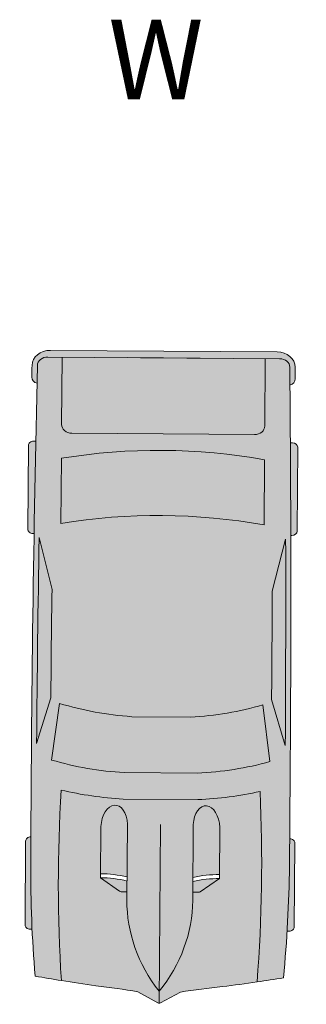
# Model space of a CAD drawing. Units: inches. Extents: x -7040 to -4088, y 6092 to 7645.
# Tile 3 of 11: x -6596 to -6542, y 6285 to 6471. Entities that reach past the tile are written whole.
import ezdxf

# ---------------------------------------------------------------- set-up
doc = ezdxf.new("R2010")
doc.units = ezdxf.units.IN
doc.layers.add('A-ANNO-TEXT', color=7, linetype='Continuous', lineweight=25)
doc.layers.add('A-SITE-VEHC', color=8, linetype='Continuous', lineweight=13)
doc.styles.get("Standard").update_dxf_attribs({"font": 'arial.ttf'})

# ---------------------------------------------------------------- blocks, each defined once
blk = doc.blocks.new('*U75')
for p, q in [((536.0433148737552, 950.1792138851854), (536.0433148737552, 935.5404748014407)), ((1182.463644577746, 987.7673041878503), (567.7039087844591, 987.7673041878503)), ((1214.124238488447, 949.7089586534819), (1214.124238488447, 950.1792138851854)), ((3440.463608272525, 941.6679440245914), (3440.463608272525, 950.1792138851854)), ((3472.124202183229, 987.7673041878503), (4086.88393797651, 987.767304187848)), ((4118.544531887212, 950.1792138851804), (4118.544531887212, 934.0601128753084)), ((2234.827175480885, 809.5287016048088), (1898.878785383111, 912.4126225124705)), ((3411.559256322833, 904.3494681924599), (3029.921878250559, 807.1504809911063)), ((1778.76917512805, 801.0177247054045), (2194.716249451875, 745.5217224176465)), ((4736.411271353851, -850.8646766016326), (4736.411271353883, 850.864676601626)), ((4785.334832293326, -832.0706314503777), (4785.334832293357, 832.0706314502926)), ((3515.941238262737, 745.5217224176508), (3994.062813016633, 745.5217224176508)), ((4736.411271353883, 745.5217224176529), (4242.012185201922, 745.5217224176529)), ((4178.690997380514, 670.345541812321), (4178.690997380509, -670.3455418123318)), ((819.5542361210883, 295.2827619512633), (917.6699264680983, 436.1082195367583)), ((917.6699264680983, 436.1082195367583), (1293.848362214069, 436.1082195367583)), ((756.2288711996046, 241.4481679439487), (1312.764151599097, 241.4481679439487)), ((815.9220749762081, 241.4481679439487), (815.9220749762081, 283.3039660446585)), ((1496.485716216861, -273.6820371142997), (1496.485716216861, 273.6820371142868)), ((1690.372337881975, -267.4332505757059), (1690.372337881975, 267.4332505756928)), ((4736.411271353883, -267.4332505757059), (4736.411271353883, 267.4332505756928)), ((82.96813941916749, 155.6585683733955), (2.596917328392246, 10.3141998552517)), ((2101.521373270556, 215.7994139342878), (2101.521373270556, -215.7994139342835)), ((-1.1252e-12, -6.4972e-12), (1312.764151599097, -6.4972e-12)), ((2.596917328392246, -10.31419985525964), (82.96813941916749, -155.6585683734063)), ((756.2288711996046, -241.4481679439617), (1312.764151599097, -241.4481679439617)), ((815.9220749762081, -241.4481679439617), (815.9220749762081, -283.3039660446715)), ((819.5542361210883, -295.2827619512763), (917.6699264680983, -436.1082195367712)), ((917.6699264680983, -436.1082195367712), (1293.848362214069, -436.1082195367712)), ((2194.716249451869, -745.5217224176688), (1778.769175128041, -801.0177247054262)), ((3994.062813016633, -745.5217224176616), (3515.941238262737, -745.5217224176638)), ((4242.012185201917, -745.5217224176638), (4736.411271353857, -745.5217224176594)), ((2234.827175480882, -809.5287016048153), (1898.878785383109, -912.4126225124726)), ((3411.559256322828, -904.349468192473), (3029.921878250557, -807.150480991115)), ((536.0433148737552, -950.1792138851984), (536.0433148737552, -935.5404748014537)), ((4118.544531887212, -950.1792138851933), (4118.544531887212, -934.0601128753214)), ((1182.463644577746, -987.7673041878633), (567.7039087844591, -987.7673041878633)), ((1214.124238488447, -949.7089586534948), (1214.124238488447, -950.1792138851984)), ((3440.463608272523, -941.6679440246044), (3440.463608272523, -950.1792138851984)), ((3472.124202183229, -987.7673041878633), (4086.883937976504, -987.767304187861))]:
    blk.add_line(p, q)
for centre, major_axis, ratio, start_param, end_param in [((1046.255263051279, -12467.92283887244), (3.2861e-12, 13417.14359589015), 0.8423038695439741, 0.0028100083536837, 0.0755983031096952), ((567.7039087844591, 950.1792138851861), (5.296e-13, -37.5880903026662), 0.842303869543976, 3.141592653589776, 4.712388980384677), ((1637.842620806017, -268112.68896731), (4.8454159e-09, 269062.8681811952), 0.842303869543847, -0.0133969486112073, 0.0027970409639888), ((1182.463644577746, 950.1792138851861), (5.601e-13, 37.58809030266621), 0.8423038695439758, -1.570796326794884, 1.73e-14), ((3472.124202183229, 950.1792138851861), (5.988e-12, -37.5880903026662), 0.8423038695439762, 3.141592653589603, 4.712388980384554), ((4086.88393797651, 950.179213885181), (1.4197e-12, 37.5880903026662), 0.842303869543976, -1.570796326794865, 4.44e-14), ((4587.952203166941, 910.2894362332722), (1.8792e-12, 56.38213545399769), 0.8423038695439691, -0.0130174256259048, 1.249894140392862), ((1637.84262086767, -268131.4830124673), (3.42859201765e-05, 269120.9512111412), 0.8423038681351471, -0.0133969484821159, -0.0130174254969711), ((4673.090083532448, 832.070631450172), (2.1733e-12, -133.2592106239272), 0.8423038695439737, 1.570796326795794, 3.128195704978164), ((6757.162543998887, -699.1204428451242), (4.9938223e-09, 7958.017136535005), 0.8423038695435286, 1.367075990158062, 1.391760499156098), ((1637.842620802809, -268112.6889680619), (4.87113144e-08, -269025.2800916445), 0.8423038695482963, 3.133765086725325, 3.140440689641252), ((4673.090083532475, 850.8646766015395), (7.5e-15, -75.17618060533067), 0.8423038695439952, 1.570796326796048, 3.128195704978389), ((3436.395912346701, 136.8410185571553), (5.76965e-11, 2077.023647078763), 0.8423038695439563, 1.245306111696802, 1.507880129813836), ((2433.035484508693, -93125.37499596032), (4.952654e-09, -93935.19844392464), 0.8423038695446962, 3.134048706297306, 3.14409775411291), ((951.8333444315502, -15086.63944974413), (1.5767e-12, -15832.53653317094), 0.8423038695439826, 3.09604606856106, 3.200911180495224), ((3413.769624379244, 136.8410185571329), (1.08602e-11, -2280.347340451234), 0.84230386954398, 4.44948196380473, 4.652344057257214), ((3799.722190048092, 71.1058404433382), (2.17448e-11, -2021.323467232052), 0.842303869543983, 4.372215489277867, 4.640744122441986), ((433.884764992104, -3.6096e-12), (1.7438e-12, 3734.255266801694), 0.8423038695439766, 4.511394369635731, 4.913383591133647), ((912.0063397460013, -3.6096e-12), (1.7438e-12, 3734.255266801694), 0.8423038695439766, 4.511394369635731, 4.913383591133647), ((4242.012185201922, 670.3455418123216), (3.5405e-12, 75.17618060533239), 0.842303869543976, 5.55e-14, 1.57079632679492), ((6583.045501169266, -699.1204428451198), (3.826807e-09, -7754.693443154298), 0.8423038695443791, 4.528606069860317, 4.561837674556238), ((-5194.164488957196, 1330.879982200552), (1.0466145e-09, -6374.389491984369), 0.8423038695441164, 1.385369446298923, 1.434372047871027), ((331.12799165183, 432.0470009052715), (3.125e-11, 696.3661584994836), 0.8423038695439277, 4.435146050259648, 4.718221029521873), ((360.7019022476185, 432.0470009052715), (3.125e-11, 696.3661584994836), 0.8423038695439277, 4.435146050259648, 4.718221029521873), ((1290.073045555822, 338.7781937403542), (161.0379696969085, -9.057857958340485), 0.6038335755719145, -1.39555193967809, 1.581314658479915), ((831.7523719315589, 283.3039660446593), (3.3347e-12, 18.79404515133458), 0.8423038695439091, 0.8797135699495516, 1.570796326795045), ((756.2288711996046, -1185.240851913765), (1.2998e-12, 1426.689019857713), 0.842303869543976, 7e-16, 0.5903187773915901), ((15.83029695535095, -3.6096e-12), (1.9e-15, -18.79404515133476), 0.842303869543842, 4.131459131953847, 5.293318828815531), ((756.2288711996046, 1185.240851913753), (1.01699e-11, 1426.689019857713), 0.8423038695439736, 2.55127387619821, 3.141592653589801), ((-5194.164488957196, -1330.879982200562), (1.0234792e-09, 6374.389491984348), 0.8423038695441192, -1.43437204787103, -1.385369446298926), ((3799.722190048497, -71.10584044329416), (1.038796e-10, -2021.323467232635), 0.8423038695439419, -1.499151468852248, -1.230622835688196), ((831.7523719315589, -283.3039660446737), (3.3028e-12, -18.79404515133458), 0.8423038695439093, 4.712388980384541, 5.403471737230034), ((331.12799165183, -432.0470009052816), (3.1922e-11, -696.3661584994801), 0.842303869543932, 1.564964277657711, 1.848039256919935), ((360.7019022476185, -432.0470009052816), (3.1922e-11, -696.3661584994801), 0.842303869543932, 1.564964277657711, 1.848039256919935), ((3413.769624379237, -136.841018557156), (1.090899e-10, -2280.347340451348), 0.8423038695439354, -1.510751403667474, -1.307889310215002), ((3436.395912346742, -136.8410185572101), (8.13766e-11, -2077.023647078826), 0.8423038695439492, -1.50788012981387, -1.245306111696839), ((6583.045501169163, 699.1204428449458), (2.756795e-10, 7754.693443157768), 0.8423038695439974, 1.721347632622872, 1.754579237318777), ((6757.162543998887, 699.1204428451076), (2.2231118e-09, 7958.017136528592), 0.8423038695441819, 1.749832154434603, 1.774516663432659), ((951.8333444315729, 15086.63944974408), (2.97009e-11, -15832.5365331709), 0.8423038695439528, -0.0593185269054384, 0.0455465850287298), ((4242.012185201917, -670.3455418123318), (2.579e-13, -75.17618060533128), 0.8423038695439885, 4.712388980384686, 6.283185307179581), ((2433.03548450906, 93125.37499596029), (4.1600574e-09, -93935.19844392457), 0.8423038695447548, -0.0025051005232382, 0.007543947292366), ((4673.090083532448, -850.8646766015358), (2.354e-13, 75.17618060532999), 0.8423038695439732, 3.154989602201626, 4.71238898038339), ((4673.090083532349, -832.0706314501077), (6.1679e-12, -133.2592106240062), 0.8423038695439807, 0.0133969486110846, 1.570796326792831), ((1046.255263051284, 12467.92283887242), (3.49903e-10, -13417.14359589015), 0.8423038695440652, -0.0755983031097181, -0.0028100083537155), ((1637.842620801787, 268112.6889680619), (1.55395844e-08, 269062.868181947), 0.8423038695458147, 3.138795612625926, 3.154989602201039), ((1637.842620803916, 268112.6889680615), (4.0766478e-08, -269025.280091644), 0.8423038695397146, 0.0011519639481523, 0.0078275668641468), ((4587.952203166856, -910.2894362333229), (5.777e-12, -56.38213545402103), 0.8423038695439803, -1.249894138785958, 0.0130174256254374), ((567.7039087844591, -950.1792138851977), (5.601e-13, 37.58809030266621), 0.8423038695439758, 1.570796326794908, 3.14159265358981), ((1182.463644577746, -950.1792138851977), (5.296e-13, -37.5880903026662), 0.842303869543976, -1.69e-14, 1.570796326794884), ((3472.124202183229, -950.1792138851955), (3.96e-13, -37.58809030266733), 0.8423038695440105, -1.570796326794875, -1.27e-14), ((4086.883937976504, -950.1792138851933), (5.0003e-12, 37.58809030266732), 0.8423038695440109, 3.141592653589951, 4.712388980384771), ((1637.842620726191, 268131.4830135791), (2.37878358395e-05, 269120.9512123862), 0.8423038705260315, 3.154610079306566, 3.154989602290631)]:
    blk.add_ellipse(centre, major_axis=major_axis, ratio=ratio, start_param=start_param, end_param=end_param)
at = {"extrusion": (0, 0, -1)}
blk.add_ellipse((1290.073045555822, -338.7781937403665), major_axis=(161.0379696969085, 9.057857958340424), ratio=0.6038335755719145, start_param=-1.39555193967809, end_param=1.581314658479915, dxfattribs=at)

msp = doc.modelspace()

# ---------------------------------------------------------------- hatches: boundary and pattern name
at = {"layer": 'A-SITE-VEHC'}
h = msp.add_hatch(color=256, dxfattribs=at)
h.dxf.hatch_style = 1
edge = h.paths.add_edge_path()
edge.add_ellipse((-13448.84234419964, 6376.78064917014), major_axis=(-6903.036062658884, 49.32613826638306), ratio=0.8423038695284738, start_angle=180.055594313474, end_angle=180.3777641938845)
edge.add_line((-6545.692544468815, 6372.968584614518), (-6548.256589051355, 6363.19380756711))
edge.add_ellipse((-8958.621342519546, 6365.100693188374), major_axis=(-2410.323900380431, 17.22314194809061), ratio=0.8423038695333621, start_angle=179.8791026309525, end_angle=180.3640763488755, ccw=False)
edge.add_line((-6548.341346917148, 6342.79169252047), (-6545.763000453511, 6334.152583520165))
edge = h.paths.add_edge_path()
edge.add_ellipse((-4179.532762243696, 6330.951373675524), major_axis=(-2410.32390038043, 17.22314194843689), ratio=0.8423038695478616, start_angle=-0.36407634889667406, end_angle=0.1208973690264088, ccw=False)
edge.add_line((-6589.678635904171, 6363.489791767677), (-6592.102733058175, 6373.300211938878))
edge.add_ellipse((310.3966401254965, 6278.463022192352), major_axis=(-6903.036062658869, 49.32613826994072), ratio=0.8423038695405606, start_angle=-0.3777641939053347, end_angle=-0.0555943134948395)
edge.add_line((-6592.586980973734, 6334.487167624397), (-6589.885441353415, 6343.088548820768))
edge = h.paths.add_edge_path()
edge.add_ellipse((-6547.315875080858, 6405.352002363618), major_axis=(-3.419355743466846, 0.0244332512076624), ratio=0.8423038695438819, start_angle=180.6465540971092, end_angle=269.9999999999045)
edge.add_line((-6547.295294858816, 6408.232138937687), (-6589.996215557602, 6408.537261422852))
edge.add_ellipse((-6590.016795779634, 6405.657124848784), major_axis=(-3.4193557434642, 0.0244332512052487), ratio=0.842303869543984, start_angle=-89.9999999999369, end_angle=-0.6465540970781114)
edge.add_ellipse((310.8788846426396, 6278.459576281303), major_axis=(-6905.490929305855, 49.34368020314359), ratio=0.8423038687222735, start_angle=-0.6465540928305886, end_angle=-0.6282372119974398)
edge.add_ellipse((-6592.039456077094, 6403.486876659906), major_axis=(-1.446733608812094, 0.0103377385495202), ratio=0.8423038695434591, start_angle=-0.6282372162717162, end_angle=68.46475660093144)
edge.add_ellipse((310.3966401062044, 6278.463022192571), major_axis=(-6904.000551712129, 49.33303009407515), ratio=0.8423038695465502, start_angle=-0.6465540970692132, end_angle=-0.6186431963266159, ccw=False)
edge.add_ellipse((-6590.499040315906, 6405.660570761636), major_axis=(-1.928978145083121, 0.0137836514007273), ratio=0.8423038695439347, start_angle=-89.99999999997772, end_angle=-0.6465540971137784, ccw=False)
edge.add_line((-6590.487430292995, 6407.285356517505), (-6546.82202052167, 6406.973342206637))
edge.add_ellipse((-6546.833630544584, 6405.348556450769), major_axis=(-1.928978145082365, 0.0137836513991165), ratio=0.8423038695438156, start_angle=180.646554097, end_angle=269.999999999814, ccw=False)
edge.add_ellipse((-13448.84234419965, 6376.780649170086), major_axis=(-6904.00055173142, 49.33303009544102), ratio=0.8423038695451385, start_angle=180.5282714718202, end_angle=180.6465540970638, ccw=False)
edge.add_ellipse((-6545.324435067654, 6403.153071133662), major_axis=(-1.446733608812857, 0.0103377385491141), ratio=0.8423038695440161, start_angle=111.535243503922, end_angle=180.6282372160688)
edge.add_ellipse((-13449.32458874532, 6376.784095081064), major_axis=(-6905.490929334866, 49.34368058577912), ratio=0.842303870966473, start_angle=180.6282372236341, end_angle=180.6465541044672)
h = msp.add_hatch(color=256, dxfattribs=at)
h.dxf.hatch_style = 1
edge = h.paths.add_edge_path()
edge.add_ellipse((-13448.84234419965, 6376.780649170086), major_axis=(-6904.00055173142, 49.33303009544102), ratio=0.8423038695451385, start_angle=180.3838667787951, end_angle=180.5282714718202)
edge.add_ellipse((-13448.84234419965, 6376.780649170086), major_axis=(-6904.00055173142, 49.33303009544102), ratio=0.8423038695451385, start_angle=180.5282714718202, end_angle=180.6465540970638)
edge.add_ellipse((-6546.833630544584, 6405.348556450769), major_axis=(-1.928978145082366, 0.0137836513991165), ratio=0.8423038695438158, start_angle=180.6465540969999, end_angle=269.9999999998141)
edge.add_line((-6546.82202052167, 6406.973342206637), (-6549.525060962446, 6406.992656975578))
edge.add_line((-6549.525060962446, 6406.992656975578), (-6549.618182154387, 6393.960642536302))
edge.add_ellipse((-6551.544687829, 6394.320440560779), major_axis=(-1.928978145082511, 0.0137836514020375), ratio=0.8423038695442027, start_angle=89.99999999999733, end_angle=179.9999999999933, ccw=False)
edge.add_line((-6551.556297851913, 6392.695654804909), (-6586.368465635523, 6392.944407641483))
edge.add_ellipse((-6585.946060428607, 6394.566258030962), major_axis=(-1.928978145083419, 0.0137836514022209), ratio=0.8423038695438055, start_angle=-1.1937117960769683e-12, end_angle=90.00000000000239, ccw=False)
edge.add_line((-6587.875038573691, 6394.580041682364), (-6587.784389852219, 6407.266041748565))
edge.add_line((-6587.784389852219, 6407.266041748565), (-6590.487430292995, 6407.285356517505))
edge.add_ellipse((-6590.499040315906, 6405.660570761636), major_axis=(-1.928978145083121, 0.0137836514007273), ratio=0.8423038695439347, start_angle=-89.99999999997772, end_angle=-0.6465540971137917)
edge.add_ellipse((310.3966401062044, 6278.463022192571), major_axis=(-6904.000551712129, 49.33303009407515), ratio=0.8423038695465502, start_angle=-0.6465540970692573, end_angle=-0.6186431963265587)
edge.add_ellipse((310.3966401062044, 6278.463022192571), major_axis=(-6904.000551712129, 49.33303009407515), ratio=0.8423038695465502, start_angle=-0.6186431963265587, end_angle=-0.5282714718252972)
edge.add_ellipse((310.3966401062044, 6278.463022192571), major_axis=(-6904.000551712129, 49.33303009407515), ratio=0.8423038695465502, start_angle=-0.5282714718252972, end_angle=-0.3838667787998605)
edge.add_ellipse((310.3966401062044, 6278.463022192571), major_axis=(-6904.000551712129, 49.33303009407515), ratio=0.8423038695465502, start_angle=-0.3838667787998605, end_angle=0.0902290885869776)
edge.add_ellipse((310.3966401062044, 6278.463022192571), major_axis=(-6904.000551712129, 49.33303009407515), ratio=0.8423038695465502, start_angle=0.0902290885869776, end_angle=0.1349865768509028)
edge.add_ellipse((-6249.411493661876, 6310.156029683172), major_axis=(-344.2762928032312, 2.460050891751548), ratio=0.8423038695443079, start_angle=0.1806905309309321, end_angle=2.179950313646397)
edge.add_ellipse((-6249.411493661876, 6310.156029683172), major_axis=(-344.2762928032312, 2.460050891751548), ratio=0.8423038695443079, start_angle=2.179950313646397, end_angle=3.650427585700186)
edge.add_ellipse((-6550.345184073126, 6458.852495946517), major_axis=(-204.1982049452834, 1.45911288418226), ratio=0.8423038695605221, start_angle=76.21947100918129, end_angle=77.87403444639521)
edge.add_ellipse((-6182.234023470371, 6307.253071690869), major_axis=(-406.2539052635208, 2.9029163576421), ratio=0.8423038695443203, start_angle=-2.1985405659517028, end_angle=2.863714607841075, ccw=False)
edge.add_ellipse((-6572.408496392596, 6373.216205047418), major_axis=(-58.51241906017842, 0.4181046783449057), ratio=0.8423038695449813, start_angle=72.28004677718432, end_angle=85.91758930878402)
edge.add_line((-6576.271295817069, 6324.044877665501), (-6562.226244205129, 6323.944517743935))
edge.add_ellipse((-6565.385970586627, 6373.166025086636), major_axis=(-58.51241906027933, 0.4181046783880361), ratio=0.8423038695435465, start_angle=94.08241069112717, end_angle=107.7199532227262)
edge.add_ellipse((-6956.463242006552, 6312.785381987249), major_axis=(-406.2539052635202, 2.902916357632984), ratio=0.8423038695434211, start_angle=177.1362853921645, end_angle=182.1985405659573, ccw=False)
edge.add_ellipse((-6586.223251944352, 6459.108865248457), major_axis=(-204.1982049532883, 1.459112884651405), ratio=0.8423038695287237, start_angle=102.1259655510788, end_angle=103.7805289882927)
edge.add_ellipse((-6889.251147049584, 6314.728049722872), major_axis=(-344.2762928032324, 2.460050891649497), ratio=0.8423038695450301, start_angle=176.3495724142852, end_angle=177.8200496863389)
edge.add_ellipse((-6889.251147049584, 6314.728049722872), major_axis=(-344.2762928032324, 2.460050891649497), ratio=0.8423038695450301, start_angle=177.8200496863389, end_angle=179.8643876095457)
edge.add_ellipse((-13448.84234419965, 6376.780649170086), major_axis=(-6904.00055173142, 49.33303009544102), ratio=0.8423038695451385, start_angle=179.8650134231458, end_angle=179.9097709114096)
edge.add_ellipse((-13448.84234419965, 6376.780649170086), major_axis=(-6904.00055173142, 49.33303009544102), ratio=0.8423038695451385, start_angle=179.9097709114096, end_angle=180.3838667787951)
edge = h.paths.add_edge_path(flags=16)
edge.add_ellipse((-4179.532762243696, 6330.951373675524), major_axis=(-2410.32390038043, 17.22314194843689), ratio=0.8423038695478616, start_angle=-0.3640763488966873, end_angle=0.120897369026304)
edge.add_line((-6589.885441353415, 6343.088548820768), (-6592.586980973734, 6334.487167624397))
edge.add_ellipse((310.3966401254965, 6278.463022192352), major_axis=(-6903.036062658869, 49.32613826994072), ratio=0.8423038695405606, start_angle=-0.3777641939053069, end_angle=-0.05559431349490751, ccw=False)
edge.add_line((-6592.102733058175, 6373.300211938878), (-6589.678635904171, 6363.489791767677))
edge = h.paths.add_edge_path(flags=16)
edge.add_line((-6574.675126462486, 6339.559136519316), (-6563.600545395731, 6339.480002307642))
edge.add_ellipse((-6567.001933054308, 6383.081401592764), major_axis=(-51.86601342390711, 0.3706123112227942), ratio=0.8423038695440606, start_angle=94.87006959713695, end_angle=112.7919148775879)
edge.add_line((-6549.991084081338, 6341.77420467811), (-6548.643352588962, 6331.091063462839))
edge.add_ellipse((-6565.381822027024, 6373.746602799445), major_axis=(-53.29524843871348, 0.3808250123157512), ratio=0.8423038695440489, start_angle=94.27742096305269, end_angle=111.8349537967064, ccw=False)
edge.add_line((-6562.351035156014, 6328.920684182548), (-6576.075406132968, 6329.018752657683))
edge.add_ellipse((-6572.404347832994, 6373.796782760226), major_axis=(-53.29524843871844, 0.3808250123137987), ratio=0.8423038695439466, start_angle=68.16504620328692, end_angle=85.72257903694049, ccw=False)
edge.add_line((-6589.750673347714, 6331.384798765569), (-6588.25041297111, 6342.047589451096))
edge.add_ellipse((-6570.651004105761, 6383.107476291133), major_axis=(-51.86601342389581, 0.370612311209319), ratio=0.842303869544027, start_angle=67.20808512239626, end_angle=85.1299304028502)
edge = h.paths.add_edge_path(flags=16)
edge.add_ellipse((-6569.443599290441, 6296.728960135292), major_axis=(-95.81887161356536, 0.6846806053339393), ratio=0.8423038695440161, start_angle=256.401865309769, end_angle=283.5981346902304)
edge.add_line((-6588.008164634965, 6375.949473101364), (-6587.920500416577, 6388.217801459713))
edge.add_ellipse((-6569.355935072055, 6308.997288493642), major_axis=(-95.81887161356295, 0.6846806053326456), ratio=0.8423038695440359, start_angle=256.4018653097682, end_angle=283.598134690229, ccw=False)
edge.add_line((-6549.661171526806, 6387.944416686727), (-6549.748835745193, 6375.676088328376))
edge = h.paths.add_edge_path(flags=16)
edge.add_ellipse((-8958.621342519546, 6365.100693188374), major_axis=(-2410.323900380431, 17.22314194809061), ratio=0.8423038695333621, start_angle=179.8791026309524, end_angle=180.3640763488755)
edge.add_line((-6548.256589051355, 6363.19380756711), (-6545.692544468815, 6372.968584614518))
edge.add_ellipse((-13448.84234419964, 6376.78064917014), major_axis=(-6903.036062658884, 49.32613826638306), ratio=0.8423038695284738, start_angle=180.0555943134741, end_angle=180.3777641938846, ccw=False)
edge.add_line((-6545.763000453511, 6334.152583520165), (-6548.341346917148, 6342.79169252047))
h = msp.add_hatch(color=256, dxfattribs=at)
h.dxf.hatch_style = 1
edge = h.paths.add_edge_path()
edge.add_line((-6549.525060962446, 6406.992656975578), (-6587.784389852219, 6407.266041748565))
edge.add_line((-6587.784389852219, 6407.266041748565), (-6587.875038573691, 6394.580041682364))
edge.add_ellipse((-6585.946060428607, 6394.566258030962), major_axis=(-1.928978145083419, 0.0137836514022209), ratio=0.8423038695438055, start_angle=-1.2645e-12, end_angle=90.00000000000242)
edge.add_line((-6585.957670451519, 6392.941472275093), (-6551.556297851913, 6392.695654804909))
edge.add_ellipse((-6551.544687829, 6394.320440560779), major_axis=(-1.928978145082511, 0.0137836514020375), ratio=0.8423038695442027, start_angle=89.99999999999719, end_angle=179.9999999999933)
edge.add_line((-6549.615709683918, 6394.306656909376), (-6549.525060962446, 6406.992656975578))
edge = h.paths.add_edge_path()
edge.add_ellipse((-6567.001933054308, 6383.081401592764), major_axis=(-51.86601342390711, 0.3706123112227942), ratio=0.8423038695440606, start_angle=94.87006959713699, end_angle=112.79191487758791, ccw=False)
edge.add_line((-6563.600545395731, 6339.480002307642), (-6574.675126462486, 6339.559136519316))
edge.add_ellipse((-6570.651004105761, 6383.107476291133), major_axis=(-51.86601342389581, 0.370612311209319), ratio=0.842303869544027, start_angle=67.20808512239631, end_angle=85.12993040285022, ccw=False)
edge.add_line((-6588.25041297111, 6342.047589451096), (-6589.750673347714, 6331.384798765569))
edge.add_ellipse((-6572.404347832994, 6373.796782760226), major_axis=(-53.29524843871844, 0.3808250123137987), ratio=0.8423038695439466, start_angle=68.16504620328683, end_angle=85.72257903694049)
edge.add_line((-6576.075406132968, 6329.018752657683), (-6562.351035156014, 6328.920684182548))
edge.add_ellipse((-6565.381822027024, 6373.746602799445), major_axis=(-53.29524843871348, 0.3808250123157512), ratio=0.8423038695440489, start_angle=94.27742096305263, end_angle=111.8349537967063)
edge.add_line((-6548.643352588962, 6331.091063462839), (-6549.991084081338, 6341.77420467811))
h = msp.add_hatch(color=256, dxfattribs=at)
h.dxf.hatch_style = 1
edge = h.paths.add_edge_path()
edge.add_ellipse((310.3966401062044, 6278.463022192571), major_axis=(-6904.000551712129, 49.33303009407515), ratio=0.8423038695465502, start_angle=-0.5282714718252919, end_angle=-0.38386677879992703, ccw=False)
edge.add_line((-6592.735464666801, 6391.446500505864), (-6593.149071653963, 6391.449455964195))
edge.add_ellipse((-6593.154876665419, 6390.63706308626), major_axis=(-0.9644890725412745, 0.0068918256984977), ratio=0.8423038695437345, start_angle=269.9999999998151, end_angle=359.9999999998435)
edge.add_line((-6594.119365737959, 6390.643954911961), (-6594.232082742547, 6374.869568859446))
edge.add_ellipse((-6593.267593670006, 6374.862677033745), major_axis=(-0.9644890725412482, 0.0068918257022932), ratio=0.8423038695437277, start_angle=6.89894e-11, end_angle=90.0000000001047)
edge.add_line((-6593.273398681462, 6374.050284155811), (-6593.055004325484, 6374.048723603308))
edge = h.paths.add_edge_path()
edge.add_ellipse((-6544.392757527737, 6390.288629873822), major_axis=(-0.9644890725412482, 0.0068918257022932), ratio=0.8423038695437277, start_angle=180.000000000069, end_angle=270.0000000001047)
edge.add_line((-6544.386952516282, 6391.101022751755), (-6544.800559503446, 6391.103978210086))
edge.add_ellipse((-13448.84234419965, 6376.780649170086), major_axis=(-6904.00055173142, 49.33303009544102), ratio=0.8423038695451385, start_angle=180.3838667787952, end_angle=180.5282714718202, ccw=False)
edge.add_line((-6544.729673899761, 6373.703411495873), (-6544.511279543782, 6373.701850943371))
edge.add_ellipse((-6544.505474532325, 6374.514243821306), major_axis=(-0.9644890725412697, 0.0068918256990648), ratio=0.8423038695446775, start_angle=89.99999999984925, end_angle=179.9999999998772)
edge.add_line((-6543.540985459784, 6374.507351995605), (-6543.428268455196, 6390.28173804812))
edge = h.paths.add_edge_path()
edge.add_ellipse((-6569.355935072055, 6308.997288493642), major_axis=(-95.81887161356295, 0.6846806053326456), ratio=0.8423038695440359, start_angle=256.4018653097682, end_angle=283.598134690229)
edge.add_line((-6587.920500416577, 6388.217801459713), (-6588.008164634965, 6375.949473101364))
edge.add_ellipse((-6569.443599290441, 6296.728960135292), major_axis=(-95.81887161356535, 0.6846806053339393), ratio=0.8423038695440161, start_angle=256.401865309769, end_angle=283.5981346902304, ccw=False)
edge.add_line((-6549.748835745193, 6375.676088328376), (-6549.661171526806, 6387.944416686727))
h = msp.add_hatch(color=256, dxfattribs=at)
h.dxf.hatch_style = 1
edge = h.paths.add_edge_path()
edge.add_line((-6575.579920085516, 6305.044396865589), (-6575.568975258241, 6306.576090609112))
edge.add_line((-6575.568975258241, 6306.576090609112), (-6576.816571588273, 6306.585005397985))
edge.add_line((-6576.816571588273, 6306.585005397985), (-6580.545186144656, 6309.222573930398))
edge.add_line((-6580.545186144656, 6309.222573930398), (-6580.476213334631, 6318.875099176593))
edge.add_ellipse((-6577.979472299618, 6318.760381104969), major_axis=(0.2619460196201628, 4.130482171573151), ratio=0.6038335755719187, start_angle=-73.65740804567889, end_angle=90.99798572499662, ccw=False)
edge.add_line((-6575.477878611259, 6319.324776424831), (-6575.579920085516, 6305.044396865589))
edge.add_ellipse((-6538.971889230861, 6304.782811560905), major_axis=(-36.60803085465607, 0.2615853046955432), ratio=0.8423038695440761, start_angle=1.57739e-11, end_angle=29.43856959799431)
edge.add_ellipse((-6599.797104919959, 6305.217442493166), major_axis=(-36.60803085465525, 0.2615853046817018), ratio=0.8423038695439949, start_angle=150.5614304020144, end_angle=179.9999999999941)
edge.add_line((-6563.189074065303, 6304.95585718848), (-6563.087032591048, 6319.236236747721))
edge.add_ellipse((-6560.593759790849, 6318.636150251858), major_axis=(-0.2028929733305537, 4.133803711868251), ratio=0.6038335755717829, start_angle=269.00201427492453, end_angle=433.6574080456019, ccw=False)
edge.add_line((-6558.095634337306, 6318.715177147481), (-6558.164607147332, 6309.062651901286))
edge.add_line((-6558.164607147332, 6309.062651901286), (-6561.930532907999, 6306.478636143129))
edge.add_line((-6561.930532907999, 6306.478636143129), (-6563.178129238028, 6306.487550932001))
edge.add_line((-6563.178129238028, 6306.487550932001), (-6563.189074065303, 6304.95585718848))
edge.add_ellipse((-6599.797104919959, 6305.217442493166), major_axis=(-36.60803085465525, 0.2615853046817018), ratio=0.8423038695439949, start_angle=150.5614304020145, end_angle=179.9999999999941, ccw=False)
edge.add_line((-6569.507140856974, 6287.836520130168), (-6569.523152631688, 6285.595723218826))
edge.add_ellipse((-6569.52025012596, 6286.001919657794), major_axis=(-0.4822445362708625, 0.0034459128493964), ratio=0.842303869544282, start_angle=89.99999999983292, end_angle=127.9331304596128)
edge.add_line((-6569.258019966692, 6285.660467522097), (-6565.513829758785, 6287.696098403654))
edge.add_ellipse((-6536.325884206272, 6152.0723906144), major_axis=(-163.5632180196099, 1.168752682009436), ratio=0.8423038695475636, start_angle=-80.74343399257413, end_angle=-77.44506735563863, ccw=False)
edge.add_ellipse((-6586.255176532723, 6454.641120710221), major_axis=(-198.9810343281642, 1.421833222596318), ratio=0.8423038695428156, start_angle=100.2095389970768, end_angle=102.4446272933776)
edge.add_ellipse((-6956.463242006552, 6312.785381987249), major_axis=(-406.2539052635202, 2.902916357632984), ratio=0.8423038695434211, start_angle=177.1362853921644, end_angle=182.1985405659573)
edge.add_ellipse((-6565.385970586627, 6373.166025086636), major_axis=(-58.51241906027933, 0.4181046783880361), ratio=0.8423038695435465, start_angle=94.08241069112711, end_angle=107.7199532227263, ccw=False)
edge.add_line((-6562.226244205129, 6323.944517743935), (-6576.271295817069, 6324.044877665501))
edge.add_ellipse((-6572.408496392596, 6373.216205047418), major_axis=(-58.51241906017842, 0.4181046783449057), ratio=0.8423038695449813, start_angle=72.28004677718428, end_angle=85.9175893087841, ccw=False)
edge.add_ellipse((-6182.234023470371, 6307.253071690869), major_axis=(-406.2539052635208, 2.9029163576421), ratio=0.8423038695443203, start_angle=-2.198540565951708, end_angle=2.863714607841071)
edge.add_ellipse((-6550.377108661503, 6454.384751408283), major_axis=(-198.9810343262183, 1.421833221154223), ratio=0.8423038695508811, start_angle=77.55537270607738, end_angle=79.79046100237807)
edge.add_ellipse((-6604.625134812547, 6152.560427798114), major_axis=(-163.5632180210948, 1.168752682151235), ratio=0.8423038695401148, start_angle=257.4450673561331, end_angle=260.74343399306883, ccw=False)
edge.add_line((-6573.502050870032, 6287.75317880936), (-6569.787333000281, 6285.664249766263))
edge.add_ellipse((-6569.52025012596, 6286.001919657794), major_axis=(-0.4822445362708625, 0.0034459128493964), ratio=0.842303869544282, start_angle=52.0668695399808, end_angle=89.99999999983292)
edge.add_line((-6569.523152631688, 6285.595723218826), (-6569.507140856974, 6287.836520130167))
edge.add_ellipse((-6538.971889230861, 6304.782811560905), major_axis=(-36.60803085465607, 0.2615853046955432), ratio=0.8423038695440761, start_angle=1.5802470443304628e-11, end_angle=29.438569597994388, ccw=False)
h = msp.add_hatch(color=256, dxfattribs=at)
h.dxf.hatch_style = 1
edge = h.paths.add_edge_path(flags=17)
edge.add_ellipse((-6577.979472299618, 6318.760381104969), major_axis=(0.2619460196201628, 4.130482171573151), ratio=0.6038335755719187, start_angle=-73.6574080456789, end_angle=90.99798572499658)
edge.add_line((-6580.476213334631, 6318.875099176593), (-6580.539763729324, 6309.981423698298))
edge.add_ellipse((-6580.543098397003, 6294.93034578045), major_axis=(-17.86836056189135, 0.127679649329033), ratio=0.8423038695431854, start_angle=251.332504507426, end_angle=270.3967098600053, ccw=False)
edge.add_line((-6575.549002158074, 6309.371262409909), (-6575.477878611259, 6319.324776424831))
edge = h.paths.add_edge_path(flags=17)
edge.add_ellipse((-6560.593759790849, 6318.636150251858), major_axis=(-0.2028929733305537, 4.133803711868251), ratio=0.6038335755717829, start_angle=269.0020142749245, end_angle=433.657408045602)
edge.add_line((-6563.087032591048, 6319.236236747721), (-6563.158156137863, 6309.282722732799))
edge.add_ellipse((-6558.370936531793, 6294.771913010873), major_axis=(-17.86836056185543, 0.1276796493424849), ratio=0.8423038695448495, start_angle=269.60329014009255, end_angle=288.66749549267456, ccw=False)
edge.add_line((-6558.159184732001, 6309.821501669186), (-6558.095634337306, 6318.715177147481))
edge = h.paths.add_edge_path()
edge.add_ellipse((-6544.925286801329, 6315.762852892491), major_axis=(-0.9644890725412736, 0.0068918256985326), ratio=0.8423038695437279, start_angle=179.9999999998456, end_angle=269.9999999998813)
edge.add_line((-6544.919481789873, 6316.575245770425), (-6544.931548272332, 6316.575331992339))
edge.add_ellipse((-13448.84234419965, 6376.780649170086), major_axis=(-6904.00055173142, 49.33303009544102), ratio=0.8423038695451385, start_angle=179.8650134231458, end_angle=179.9097709114097, ccw=False)
edge.add_ellipse((-6889.251147049584, 6314.728049722872), major_axis=(-344.2762928032324, 2.460050891649497), ratio=0.8423038695450301, start_angle=177.8200496863389, end_angle=179.8643876095458, ccw=False)
edge.add_line((-6545.419430557354, 6299.178757994068), (-6545.043808817371, 6299.176073962041))
edge.add_ellipse((-6545.038003805915, 6299.988466839976), major_axis=(-0.964489072541239, 0.0068918257035405), ratio=0.8423038695446706, start_angle=90.00000000017933, end_angle=180.000000000143)
edge.add_line((-6544.073514733374, 6299.981575014275), (-6543.960797728786, 6315.755961066789))
edge = h.paths.add_edge_path()
edge.add_ellipse((-6249.411493661876, 6310.156029683172), major_axis=(-344.2762928032312, 2.460050891751548), ratio=0.8423038695443079, start_angle=0.13561239043957585, end_angle=0.1806905309309741, ccw=False)
edge.add_ellipse((310.3966401062044, 6278.463022192571), major_axis=(-6904.000551712129, 49.33303009407515), ratio=0.8423038695465502, start_angle=0.09022908858702294, end_angle=0.1349865768509062, ccw=False)
edge.add_line((-6593.669534445095, 6316.92359276095), (-6593.681600927553, 6316.923678982863))
edge.add_ellipse((-6593.687405939007, 6316.11128610493), major_axis=(-0.9644890725421756, 0.0068918256995869), ratio=0.8423038695429337, start_angle=269.9999999999436, end_angle=359.9999999999082)
edge.add_line((-6594.65189501155, 6316.118177930631), (-6594.764612016136, 6300.343791878114))
edge.add_ellipse((-6593.800122943595, 6300.336900052414), major_axis=(-0.9644890725412778, 0.006891825697266), ratio=0.8423038695446834, start_angle=-1.756348e-10, end_angle=89.99999999974241)
edge.add_line((-6593.805927955052, 6299.52450717448), (-6593.430306215072, 6299.521823142452))
edge.add_ellipse((-6249.411493661876, 6310.156029683172), major_axis=(-344.2762928032312, 2.460050891751548), ratio=0.8423038695443079, start_angle=0.1806905309309741, end_angle=2.1799503136463727, ccw=False)
edge = h.paths.add_edge_path(flags=17)
edge.add_ellipse((-6560.593759790849, 6318.636150251858), major_axis=(-0.2028929733305537, 4.133803711868251), ratio=0.6038335755717829, start_angle=269.0020142749245, end_angle=433.657408045602)
edge.add_line((-6563.087032591048, 6319.236236747721), (-6563.158156137863, 6309.282722732799))
edge.add_ellipse((-6558.370936531793, 6294.771913010873), major_axis=(-17.86836056185543, 0.1276796493424849), ratio=0.8423038695448495, start_angle=269.60329014009255, end_angle=288.66749549267456, ccw=False)
edge.add_line((-6558.159184732001, 6309.821501669186), (-6558.095634337306, 6318.715177147481))
edge = h.paths.add_edge_path(flags=17)
edge.add_ellipse((-6577.979472299618, 6318.760381104969), major_axis=(0.2619460196201628, 4.130482171573151), ratio=0.6038335755719187, start_angle=-73.6574080456789, end_angle=90.99798572499658)
edge.add_line((-6580.476213334631, 6318.875099176593), (-6580.539763729324, 6309.981423698298))
edge.add_ellipse((-6580.543098397003, 6294.93034578045), major_axis=(-17.86836056189135, 0.127679649329033), ratio=0.8423038695431854, start_angle=251.332504507426, end_angle=270.3967098600053, ccw=False)
edge.add_line((-6575.549002158074, 6309.371262409909), (-6575.477878611259, 6319.324776424831))
h = msp.add_hatch(color=256, dxfattribs=at)
h.dxf.hatch_style = 1
edge = h.paths.add_edge_path()
edge.add_ellipse((-6560.593759790849, 6318.636150251858), major_axis=(-0.2028929733305537, 4.133803711868251), ratio=0.6038335755717829, start_angle=269.0020142749245, end_angle=433.657408045602)
edge.add_line((-6563.087032591048, 6319.236236747721), (-6563.158156137863, 6309.282722732799))
edge.add_ellipse((-6558.370936531793, 6294.771913010873), major_axis=(-17.86836056185543, 0.1276796493424849), ratio=0.8423038695448495, start_angle=269.60329014009255, end_angle=288.66749549267456, ccw=False)
edge.add_line((-6558.159184732001, 6309.821501669186), (-6558.095634337306, 6318.715177147481))
edge = h.paths.add_edge_path()
edge.add_ellipse((-6580.548520812334, 6294.171496012551), major_axis=(-17.86836056186519, 0.1276796493187718), ratio=0.8423038695444228, start_angle=251.3325045073925, end_angle=270.3967098599764)
edge.add_line((-6580.545186144656, 6309.222573930398), (-6576.949674437303, 6306.679160446963))
edge.add_ellipse((-6576.640068785978, 6306.989961363608), major_axis=(-0.4822445362643308, 0.003445912835244), ratio=0.8423038695539805, start_angle=45.51978911553989, end_angle=89.99999999815618)
edge.add_line((-6576.642971291708, 6306.58376492464), (-6575.568975258241, 6306.576090609112))
edge.add_line((-6575.568975258241, 6306.576090609112), (-6575.554424573406, 6308.612412642009))
edge = h.paths.add_edge_path()
edge.add_ellipse((-6577.979472299618, 6318.760381104969), major_axis=(0.2619460196201628, 4.130482171573151), ratio=0.6038335755719187, start_angle=-73.6574080456789, end_angle=90.99798572499658)
edge.add_line((-6580.476213334631, 6318.875099176593), (-6580.539763729324, 6309.981423698298))
edge.add_ellipse((-6580.543098397003, 6294.93034578045), major_axis=(-17.86836056189135, 0.127679649329033), ratio=0.8423038695431854, start_angle=251.332504507426, end_angle=270.3967098600053, ccw=False)
edge.add_line((-6575.549002158074, 6309.371262409909), (-6575.477878611259, 6319.324776424831))
edge = h.paths.add_edge_path()
edge.add_ellipse((-6558.376358947123, 6294.013063242974), major_axis=(-17.86836056188143, 0.1276796493111785), ratio=0.8423038695436819, start_angle=269.6032901399951, end_angle=288.6674954925736)
edge.add_line((-6563.163578553193, 6308.523872964899), (-6563.178129238028, 6306.487550932001))
edge.add_line((-6563.178129238028, 6306.487550932001), (-6562.104133204562, 6306.479876616474))
edge.add_ellipse((-6562.101230698835, 6306.886073055441), major_axis=(-0.4822445362724531, 0.003445912845044), ratio=0.8423038695415588, start_angle=89.99999999931448, end_angle=134.4802108819163)
edge.add_line((-6561.796098135943, 6306.570879482884), (-6558.164607147332, 6309.062651901286))

# ---------------------------------------------------------------- block references
at = {"layer": 'A-SITE-VEHC', "xscale": 0.0256600877426223, "yscale": 0.0256600877426223, "zscale": 0.0256600877426223, "rotation": 89.59059587440655}
msp.add_blockref('*U75', (-6569.523152631688, 6285.595723218826), dxfattribs=at)

# ---------------------------------------------------------------- texts
at = {"layer": 'A-ANNO-TEXT', "insert": (-6579.095400825028, 6470.810245072178), "char_height": 15, "attachment_point": 1}
msp.add_mtext_dynamic_manual_height_columns('{W}', width=701.5203491572992, gutter_width=12.5, heights=[0], dxfattribs=at)

doc.saveas('drawing.dxf')
